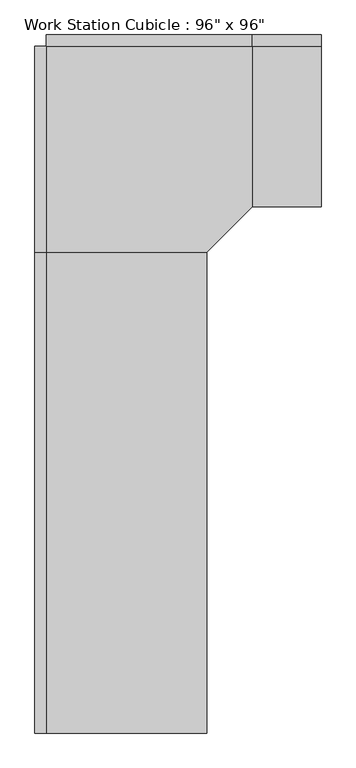
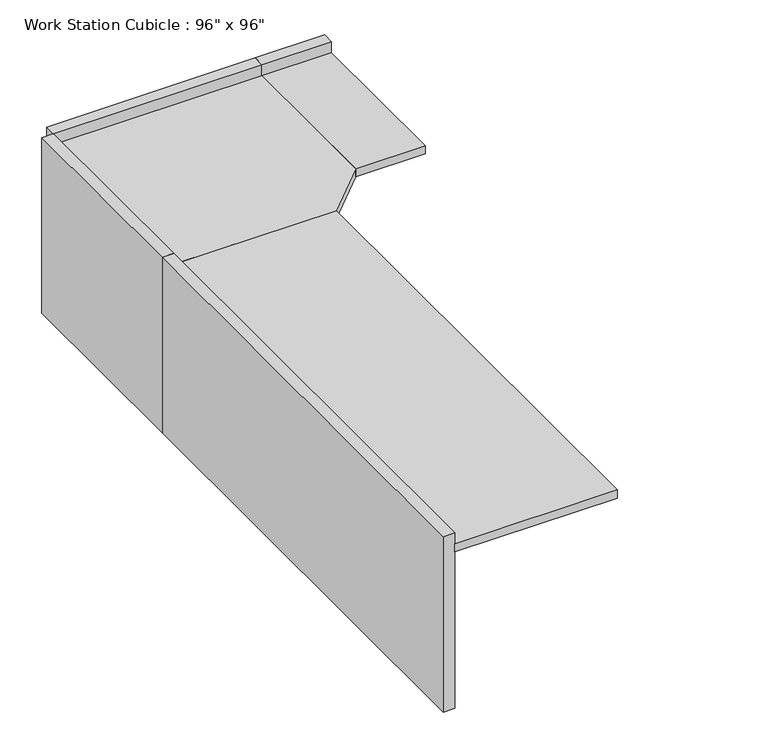
"""IFC4 building model written with IfcOpenShell, lengths in millimetres: furniture geometry."""

from ifc_helpers import new_model, si_unit, frame, origin, origin_with_axes, place, context, project, spatial, polyline, outline, extrude, source, transform, mapped, element, save


def furniture_8edce76a(model_context):
    return source(origin(), model_context, "Body", "SweptSolid", [
        extrude(outline(polyline([(-80.9317522, -545.8230076), (833.4682478, -545.8230076), (833.4682478, -1257.0230076), (630.2682478, -1460.2230076), (-80.9317522, -1460.2230076), (-80.9317522, -545.8230076)])), frame((0.0, 0.0, 723.9), z_axis=(0.0, 0.0, 1.0), x_axis=(1.0, 0.0, 0.0)), (0.0, 0.0, 1.0), 38.1),
        extrude(outline(polyline([(630.2682478, -3593.8230076), (-80.9317522, -3593.8230076), (-80.9317522, -1460.2230076), (630.2682478, -1460.2230076), (630.2682478, -3593.8230076)])), frame((0.0, 0.0, 723.9), z_axis=(0.0, 0.0, 1.0), x_axis=(1.0, 0.0, 0.0)), (0.0, 0.0, 1.0), 38.1),
        extrude(outline(polyline([(1138.2682478, -1257.0230076), (833.4682478, -1257.0230076), (833.4682478, -545.8230076), (1138.2682478, -545.8230076), (1138.2682478, -1257.0230076)])), frame((0.0, 0.0, 723.9), z_axis=(0.0, 0.0, 1.0), x_axis=(1.0, 0.0, 0.0)), (0.0, 0.0, 1.0), 38.1),
        extrude(outline(polyline([(1138.2682478, -545.8230076), (833.4682478, -545.8230076), (833.4682478, -495.0230076), (1138.2682478, -495.0230076), (1138.2682478, -545.8230076)])), origin_with_axes(), (0.0, 0.0, 1.0), 812.8),
        extrude(outline(polyline([(833.4682478, -545.8230076), (-80.9317522, -545.8230076), (-80.9317522, -495.0230076), (833.4682478, -495.0230076), (833.4682478, -545.8230076)])), origin_with_axes(), (0.0, 0.0, 1.0), 812.8),
        extrude(outline(polyline([(-80.9317522, -1460.2230076), (-131.7317522, -1460.2230076), (-131.7317522, -545.8230076), (-80.9317522, -545.8230076), (-80.9317522, -1460.2230076)])), origin_with_axes(), (0.0, 0.0, 1.0), 812.8),
        extrude(outline(polyline([(-80.9317522, -3593.8230076), (-131.7317522, -3593.8230076), (-131.7317522, -1460.2230076), (-80.9317522, -1460.2230076), (-80.9317522, -3593.8230076)])), origin_with_axes(), (0.0, 0.0, 1.0), 812.8),
    ])


if __name__ == "__main__":
    model = new_model("IFC4")
    model_context = context("Model", 3, world=origin())
    ifc_project = project(units=[si_unit("LENGTHUNIT", "METRE", prefix="MILLI")], contexts=[model_context])
    site = spatial("IfcSite", under=ifc_project)
    building = spatial("IfcBuilding", under=site)
    placement = place(None, origin())
    furniture_shape = furniture_8edce76a(model_context)
    element("IfcFurniture", 1, ObjectType="Work Station Cubicle : 96\" x 96\"", at=placement, inside=building, context=model_context, shape_type="MappedRepresentation", body=[
        mapped(furniture_shape, transform((0.0, 0.0, 0.0), x_axis=(1.0, 0.0, 0.0), y_axis=(0.0, 1.0, 0.0), z_axis=(0.0, 0.0, 1.0))),
    ])
    save(model, "model.ifc")

# Revit data of these elements
# Type "Work Station Cubicle : 96\" x 96\""
#   Assembly Code = "E2020"
#   Desktop Height = 2' - 6"
#   Desktop1 Width = 2' - 4"
#   Desktop2 Width = 2' - 4"
#   Panel Height = 2' - 8"
#   Panel1 Length = 7' - 0"
#   Panel2 Length = 1' - 0"
#   Cube Panel Material = Textile - Light Gray
#   Work Top Material = Laminate, Ivory, Matte
#   Default Elevation = 0
# Element 1 (IfcFurniture, "Work Station Cubicle : 96\" x 96\"")
#   Materials on its faces: "Textile - Light Gray", "Laminate, Ivory, Matte"
# Materials
#   "Textile - Light Gray": class "Fabric", colour RGB 204 204 204, transparency 0
#   "Laminate, Ivory, Matte": class "Plastic", colour RGB 247 247 239, transparency 0, Description = "Plastic Laminate - Ivory, Matte", Cost = 0
